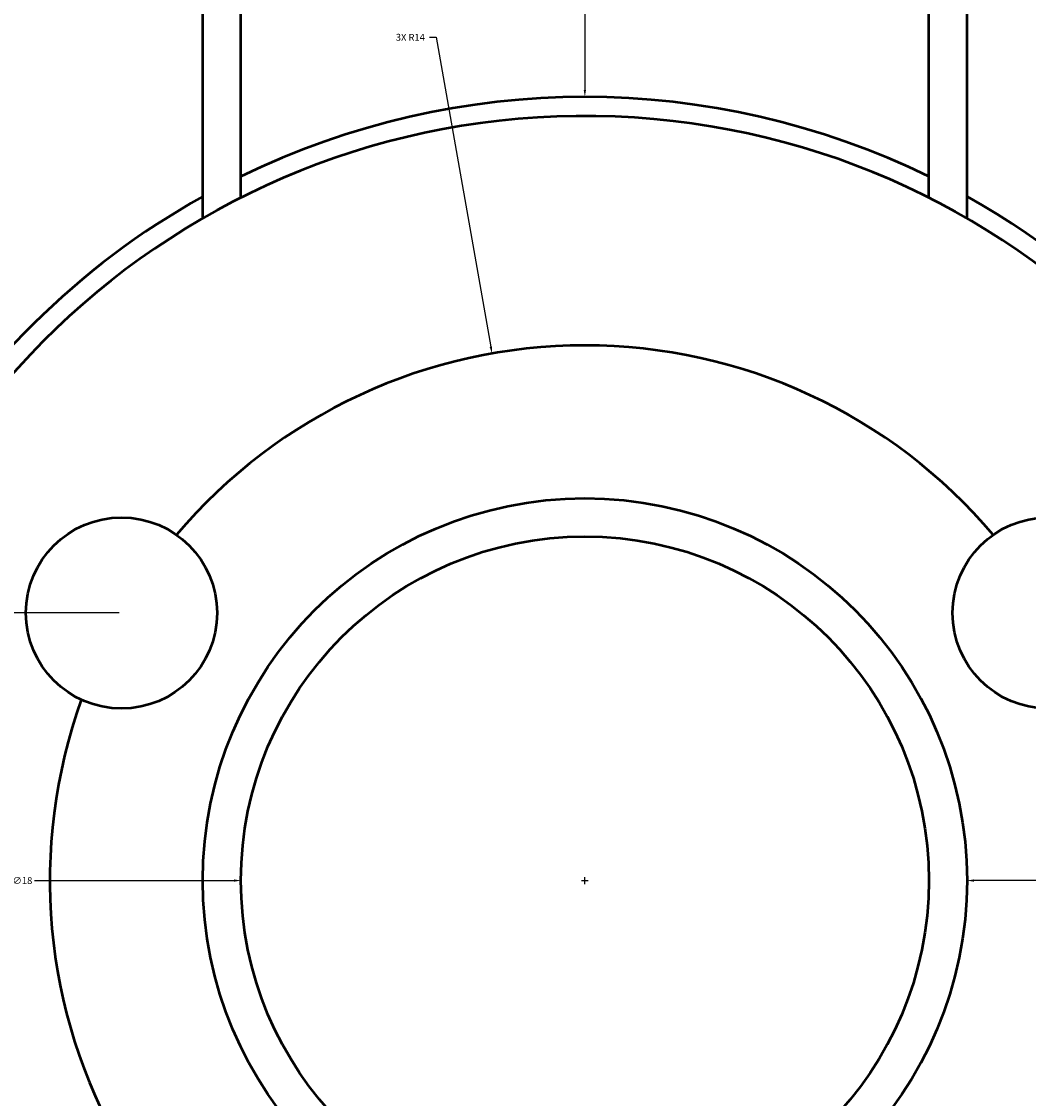
# Model space of a CAD drawing. Units: inches. Extents: x -19.9 to 72.3, y -39.8 to 57.5.
# Tile 5 of 8: x 13.3 to 39.7, y 7.6 to 35.8. Entities that reach past the tile are written whole.
import ezdxf

# ---------------------------------------------------------------- set-up
doc = ezdxf.new("R2010")
doc.units = ezdxf.units.IN
doc.header["$MEASUREMENT"] = 0
for name, color, linetype, lineweight in [('M-DIMS', 2, 'Continuous', 18), ('M-OUTL', 7, 'Continuous', 50), ('M-OUTL-HOLE', 7, 'Continuous', 50), ('M-OUTL-SLOT', 7, 'Continuous', 50)]:
    doc.layers.add(name, color=color, linetype=linetype, lineweight=lineweight)
doc.styles.get("Standard").update_dxf_attribs({"font": 'arial.ttf'})
doc.dimstyles.get("Standard").update_dxf_attribs({"dimtxt": 0.18, "dimasz": 0.18, "dimexe": 0.18, "dimexo": 0.0625, "dimgap": 0.09, "dimtad": 0, "dimtih": 1, "dimtoh": 1, "dimdec": 4, "dimzin": 0, "dimdsep": 46, "dimtxsty": 'Standard', "dimcen": 0.09, "dimadec": 0, "dimazin": 0, "dimtfac": 1, "dimtdec": 4, "dimtofl": 0, "dimtmove": 0, "dimatfit": 3, "dimfxl": 1, "dimtolj": 1, "dimtzin": 0, "dimarcsym": 0})

# ---------------------------------------------------------------- blocks, each defined once
blk = doc.blocks.new('FLANGE-MOUNT-D8-RELIEVED')
for start, end in [(109.4712, 138.6562), (161.3438, 190.5288)]:
    blk.add_arc((26.414, -15.25), 30, start, end)
blk = doc.blocks.new('HUB-HOLE-D5')
blk.add_circle((0, 0), 2.5)
blk = doc.blocks.new('FLANGE-STRAIGHT-SLOT')
for p, q in [((0, 0), (0, 21.114)), ((1, -0.54), (1, 20.869))]:
    blk.add_line(p, q)
blk = doc.blocks.new('*D6')
at = {"layer": 'Defpoints', "color": 0, "transparency": 16777216}
for p in [(28.06, 43.841), (28.06, -17.159), (72.086, -17.159)]:
    blk.add_point(p, dxfattribs=at)
at = {"layer": 'M-DIMS', "color": 0, "lineweight": -2, "transparency": 16777216}
for p, q in [((28.122, 43.841), (72.266, 43.841)), ((72.086, 43.661), (72.086, 13.523)), ((72.086, -16.979), (72.086, 13.159)), ((28.122, -17.159), (72.266, -17.159))]:
    blk.add_line(p, q, dxfattribs=at)
at = {"layer": 'M-DIMS', "color": 0, "transparency": 16777216}
for points in [[(72.056, 43.661), (72.116, 43.661), (72.086, 43.841)], [(72.056, -16.979), (72.116, -16.979), (72.086, -17.159)]]:
    blk.add_solid(points, dxfattribs=at)
at = {"layer": 'M-DIMS', "color": 0, "transparency": 16777216, "insert": (72.086, 13.341), "char_height": 0.18, "attachment_point": 5}
blk.add_mtext('\\A1;61', dxfattribs=at)
blk = doc.blocks.new('*D9')
at = {"layer": 'Defpoints', "color": 0, "transparency": 16777216}
for p in [(15.936, 20.341), (-15.966, -0.659), (28.06, -0.659)]:
    blk.add_point(p, dxfattribs=at)
at = {"layer": 'M-DIMS', "color": 0, "lineweight": -2, "transparency": 16777216}
for p, q in [((15.873, 20.341), (-16.146, 20.341)), ((-15.966, 20.161), (-15.966, 10.022)), ((-15.966, -0.479), (-15.966, 9.661)), ((27.997, -0.659), (-16.146, -0.659))]:
    blk.add_line(p, q, dxfattribs=at)
at = {"layer": 'M-DIMS', "color": 0, "transparency": 16777216}
for points in [[(-15.996, 20.161), (-15.936, 20.161), (-15.966, 20.341)], [(-15.996, -0.479), (-15.936, -0.479), (-15.966, -0.659)]]:
    blk.add_solid(points, dxfattribs=at)
at = {"layer": 'M-DIMS', "color": 0, "transparency": 16777216, "insert": (-15.966, 9.841), "char_height": 0.18, "attachment_point": 5}
blk.add_mtext('\\A1;21', dxfattribs=at)
blk = doc.blocks.new('*D10')
at = {"layer": 'Defpoints', "color": 0, "transparency": 16777216}
for p in [(28.06, 43.841), (-15.966, 28.591), (1.646, 28.591)]:
    blk.add_point(p, dxfattribs=at)
at = {"layer": 'M-DIMS', "color": 0, "lineweight": -2, "transparency": 16777216}
for p, q in [((27.997, 43.841), (-16.146, 43.841)), ((-15.966, 43.661), (-15.966, 36.398)), ((-15.966, 28.771), (-15.966, 36.034)), ((1.584, 28.591), (-16.146, 28.591))]:
    blk.add_line(p, q, dxfattribs=at)
at = {"layer": 'M-DIMS', "color": 0, "transparency": 16777216}
for points in [[(-15.996, 43.661), (-15.936, 43.661), (-15.966, 43.841)], [(-15.996, 28.771), (-15.936, 28.771), (-15.966, 28.591)]]:
    blk.add_solid(points, dxfattribs=at)
at = {"layer": 'M-DIMS', "color": 0, "transparency": 16777216, "insert": (-15.966, 36.216), "char_height": 0.18, "attachment_point": 5}
blk.add_mtext('\\A1;15.25', dxfattribs=at)
blk = doc.blocks.new('*D11')
at = {"layer": 'Defpoints', "color": 0, "transparency": 16777216}
for p in [(5.703, 46.51), (50.417, -19.828)]:
    blk.add_point(p, dxfattribs=at)
at = {"layer": 'M-DIMS', "color": 0, "lineweight": -2, "transparency": 16777216}
for p, q in [((27.97, 13.341), (28.15, 13.341)), ((28.06, 13.251), (28.06, 13.431)), ((63.831, -39.729), (50.517, -19.977)), ((64.011, -39.729), (63.831, -39.729))]:
    blk.add_line(p, q, dxfattribs=at)
at = {"layer": 'M-DIMS', "color": 0, "transparency": 16777216}
blk.add_solid([(50.542, -19.96), (50.492, -19.994), (50.417, -19.828)], dxfattribs=at)
at = {"layer": 'M-DIMS', "color": 0, "transparency": 16777216, "insert": (64.327, -39.729), "char_height": 0.18, "attachment_point": 5}
blk.add_mtext('\\A1;∅80', dxfattribs=at)
blk = doc.blocks.new('*D12')
at = {"layer": 'Defpoints', "color": 0, "transparency": 16777216}
for p in [(28.06, 13.341), (-1.285, 3.349)]:
    blk.add_point(p, dxfattribs=at)
at = {"layer": 'M-DIMS', "color": 0, "lineweight": -2, "transparency": 16777216}
for p, q in [((27.97, 13.341), (28.15, 13.341)), ((28.06, 13.251), (28.06, 13.431)), ((-18.893, -2.647), (-1.456, 3.291)), ((-19.073, -2.647), (-18.893, -2.647))]:
    blk.add_line(p, q, dxfattribs=at)
at = {"layer": 'M-DIMS', "color": 0, "transparency": 16777216}
blk.add_solid([(-1.466, 3.319), (-1.446, 3.262), (-1.285, 3.349)], dxfattribs=at)
at = {"layer": 'M-DIMS', "color": 0, "transparency": 16777216, "insert": (-19.557, -2.647), "char_height": 0.18, "attachment_point": 5}
blk.add_mtext('\\A1;4X R31', dxfattribs=at)
blk = doc.blocks.new('*D13')
at = {"layer": 'Defpoints', "color": 0, "transparency": 16777216}
for p in [(11.256, 38.194), (28.06, 13.341)]:
    blk.add_point(p, dxfattribs=at)
at = {"layer": 'M-DIMS', "color": 0, "lineweight": -2, "transparency": 16777216}
for p, q in [((0.994, 53.105), (1.174, 53.105)), ((1.174, 53.105), (11.155, 38.343)), ((27.97, 13.341), (28.15, 13.341)), ((28.06, 13.251), (28.06, 13.431))]:
    blk.add_line(p, q, dxfattribs=at)
at = {"layer": 'M-DIMS', "color": 0, "transparency": 16777216}
blk.add_solid([(11.18, 38.36), (11.131, 38.326), (11.256, 38.194)], dxfattribs=at)
at = {"layer": 'M-DIMS', "color": 0, "transparency": 16777216, "insert": (0.434, 53.105), "char_height": 0.18, "attachment_point": 5}
blk.add_mtext('\\A1;10X R30', dxfattribs=at)
blk = doc.blocks.new('*D14')
at = {"layer": 'Defpoints', "color": 0, "transparency": 16777216}
for p in [(28.06, 33.841), (28.06, 13.341)]:
    blk.add_point(p, dxfattribs=at)
at = {"layer": 'M-DIMS', "color": 0, "lineweight": -2, "transparency": 16777216}
for p, q in [((28.24, 46.141), (28.06, 46.141)), ((28.06, 46.141), (28.06, 34.021)), ((27.97, 13.341), (28.15, 13.341)), ((28.06, 13.251), (28.06, 13.431))]:
    blk.add_line(p, q, dxfattribs=at)
at = {"layer": 'M-DIMS', "color": 0, "transparency": 16777216}
blk.add_solid([(28.03, 34.021), (28.09, 34.021), (28.06, 33.841)], dxfattribs=at)
at = {"layer": 'M-DIMS', "color": 0, "transparency": 16777216, "insert": (28.844, 46.141), "char_height": 0.18, "attachment_point": 5}
blk.add_mtext('\\A1;3X R20.5', dxfattribs=at)
blk = doc.blocks.new('*D15')
at = {"layer": 'Defpoints', "color": 0, "transparency": 16777216}
for p in [(12.739, 26.197), (28.06, 13.341)]:
    blk.add_point(p, dxfattribs=at)
at = {"layer": 'M-DIMS', "color": 0, "lineweight": -2, "transparency": 16777216}
for p, q in [((3.366, 33.91), (3.546, 33.91)), ((3.546, 33.91), (12.601, 26.313)), ((27.97, 13.341), (28.15, 13.341)), ((28.06, 13.251), (28.06, 13.431))]:
    blk.add_line(p, q, dxfattribs=at)
at = {"layer": 'M-DIMS', "color": 0, "transparency": 16777216}
blk.add_solid([(12.62, 26.336), (12.582, 26.29), (12.739, 26.197)], dxfattribs=at)
at = {"layer": 'M-DIMS', "color": 0, "transparency": 16777216, "insert": (3.062, 33.91), "char_height": 0.18, "attachment_point": 5}
blk.add_mtext('\\A1;R20', dxfattribs=at)
blk = doc.blocks.new('*D16')
at = {"layer": 'Defpoints', "color": 0, "transparency": 16777216}
for p in [(25.629, 27.129), (28.06, 13.341)]:
    blk.add_point(p, dxfattribs=at)
at = {"layer": 'M-DIMS', "color": 0, "lineweight": -2, "transparency": 16777216}
for p, q in [((23.991, 35.401), (24.171, 35.401)), ((24.171, 35.401), (25.598, 27.306)), ((27.97, 13.341), (28.15, 13.341)), ((28.06, 13.251), (28.06, 13.431))]:
    blk.add_line(p, q, dxfattribs=at)
at = {"layer": 'M-DIMS', "color": 0, "transparency": 16777216}
blk.add_solid([(25.627, 27.311), (25.568, 27.301), (25.629, 27.129)], dxfattribs=at)
at = {"layer": 'M-DIMS', "color": 0, "transparency": 16777216, "insert": (23.493, 35.401), "char_height": 0.18, "attachment_point": 5}
blk.add_mtext('\\A1;3X R14', dxfattribs=at)
blk = doc.blocks.new('*D18')
at = {"layer": 'Defpoints', "color": 0, "transparency": 16777216}
for p in [(18.06, 13.342), (38.06, 13.341)]:
    blk.add_point(p, dxfattribs=at)
at = {"layer": 'M-DIMS', "color": 0, "lineweight": -2, "transparency": 16777216}
for p, q in [((27.97, 13.341), (28.15, 13.341)), ((28.06, 13.251), (28.06, 13.431)), ((44.06, 13.341), (38.24, 13.341))]:
    blk.add_line(p, q, dxfattribs=at)
at = {"layer": 'M-DIMS', "color": 0, "transparency": 16777216}
blk.add_solid([(38.24, 13.371), (38.24, 13.311), (38.06, 13.341)], dxfattribs=at)
at = {"layer": 'M-DIMS', "color": 0, "transparency": 16777216, "insert": (44.376, 13.341), "char_height": 0.18, "attachment_point": 5}
blk.add_mtext('\\A1;∅20', dxfattribs=at)
blk = doc.blocks.new('*D19')
at = {"layer": 'Defpoints', "color": 0, "transparency": 16777216}
for p in [(19.06, 13.341), (37.06, 13.342)]:
    blk.add_point(p, dxfattribs=at)
at = {"layer": 'M-DIMS', "color": 0, "lineweight": -2, "transparency": 16777216}
for p, q in [((13.66, 13.341), (18.88, 13.341)), ((27.97, 13.341), (28.15, 13.341)), ((28.06, 13.251), (28.06, 13.431))]:
    blk.add_line(p, q, dxfattribs=at)
at = {"layer": 'M-DIMS', "color": 0, "transparency": 16777216}
blk.add_solid([(18.88, 13.371), (18.88, 13.311), (19.06, 13.341)], dxfattribs=at)
at = {"layer": 'M-DIMS', "color": 0, "transparency": 16777216, "insert": (13.343, 13.341), "char_height": 0.18, "attachment_point": 5}
blk.add_mtext('\\A1;∅18', dxfattribs=at)

msp = doc.modelspace()

# ---------------------------------------------------------------- linework, layer by layer
at = {"layer": 'M-OUTL'}
for radius in [40, 10, 9]:
    msp.add_circle((28.06, 13.341), radius, dxfattribs=at)
for radius, start, end in [(20.5, 63.9584, 116.0416), (20, 0, 356.7437), (20.5, 119.1964, 180.8036), (20.5, 183.9584, 60.8036), (14, 40.245, 139.755), (14, 160.245, 259.755), (14, 280.245, 19.755)]:
    msp.add_arc((28.06, 13.341), radius, start, end, dxfattribs=at)

# ---------------------------------------------------------------- block references
at = {"layer": 'M-OUTL-HOLE', "rotation": 240}
msp.add_blockref('FLANGE-MOUNT-D8-RELIEVED', (54.474, 28.591), dxfattribs=at)
at = {"layer": 'M-OUTL-HOLE'}
for name, p in [('FLANGE-MOUNT-D8-RELIEVED', (1.646, 28.591)), ('HUB-HOLE-D5', (15.936, 20.341)), ('HUB-HOLE-D5', (40.184, 20.341))]:
    msp.add_blockref(name, p, dxfattribs=at)
at = {"layer": 'M-OUTL-SLOT', "extrusion": (0, 0, -1), "zscale": -1}
msp.add_blockref('FLANGE-STRAIGHT-SLOT', (-19.06, 31.202), dxfattribs=at)
at = {"layer": 'M-OUTL-SLOT'}
msp.add_blockref('FLANGE-STRAIGHT-SLOT', (37.06, 31.202), dxfattribs=at)

# ---------------------------------------------------------------- dimensions: what is measured, and where the dimension line sits
at = {"layer": 'M-DIMS'}
for mpoint, text, override, picture, middle in [((11.256, 38.194), '10X <>', {"dimdec": 0, "dimlfac": 1, "dimrnd": 0, "dimzin": 0, "dimdsep": 46, "dimlunit": 2}, '*D13', (0.434, 53.105)), ((28.06, 33.841), '3X <>', {"dimdec": 1, "dimlfac": 1, "dimrnd": 0, "dimzin": 0, "dimdsep": 46, "dimlunit": 2}, '*D14', (28.844, 46.141)), ((25.629, 27.129), '3X <>', {"dimdec": 0, "dimlfac": 1, "dimrnd": 0, "dimzin": 0, "dimdsep": 46, "dimlunit": 2}, '*D16', (23.493, 35.401)), ((-1.285, 3.349), '4X <>', {"dimdec": 0, "dimlfac": 1, "dimrnd": 0, "dimzin": 0, "dimdsep": 46, "dimlunit": 2}, '*D12', (-19.557, -2.647))]:
    dim = msp.add_radius_dim(center=(28.06, 13.341), mpoint=mpoint, text=text, dimstyle='Standard', override=override, dxfattribs=at)
    dim.commit()
    dim.dimension.update_dxf_attribs({"geometry": picture, "text_midpoint": middle, "dimtype": 164})
for p1, p2, picture, middle in [((5.703, 46.51), (50.417, -19.828), '*D11', (64.327, -39.729)), ((37.06, 13.342), (19.06, 13.341), '*D19', (13.66, 13.341)), ((18.06, 13.342), (38.06, 13.341), '*D18', (44.06, 13.341))]:
    dim = msp.add_diameter_dim_2p(p1=p1, p2=p2, dimstyle='Standard', override={"dimdec": 0, "dimlfac": 1, "dimrnd": 0, "dimzin": 0, "dimdsep": 46, "dimlunit": 2}, dxfattribs=at)
    dim.commit()
    dim.dimension.update_dxf_attribs({"geometry": picture, "text_midpoint": middle, "dimtype": 163})
for base, p1, p2, override, picture, middle in [((-15.966, 28.591), (28.06, 43.841), (1.646, 28.591), {"dimdec": 2, "dimlfac": 1, "dimrnd": 0, "dimzin": 0, "dimdsep": 46, "dimlunit": 2}, '*D10', (-15.966, 36.216)), ((72.086, -17.159), (28.06, 43.841), (28.06, -17.159), {"dimdec": 0, "dimlfac": 1, "dimrnd": 0, "dimzin": 0, "dimdsep": 46, "dimlunit": 2}, '*D6', (72.086, 13.341)), ((-15.966, -0.659), (15.936, 20.341), (28.06, -0.659), {"dimdec": 0, "dimlfac": 1, "dimrnd": 0, "dimzin": 0, "dimdsep": 46, "dimlunit": 2}, '*D9', (-15.966, 9.841))]:
    dim = msp.add_linear_dim(base=base, p1=p1, p2=p2, angle=90, dimstyle='Standard', override=override, dxfattribs=at)
    dim.commit()
    dim.dimension.update_dxf_attribs({"geometry": picture, "text_midpoint": middle})
dim = msp.add_radius_dim(center=(28.06, 13.341), mpoint=(12.739, 26.197), dimstyle='Standard', override={"dimdec": 0, "dimlfac": 1, "dimrnd": 0, "dimzin": 0, "dimdsep": 46, "dimlunit": 2}, dxfattribs=at)
dim.commit()
dim.dimension.update_dxf_attribs({"geometry": '*D15', "text_midpoint": (3.062, 33.91), "dimtype": 164})

doc.saveas('drawing.dxf')
